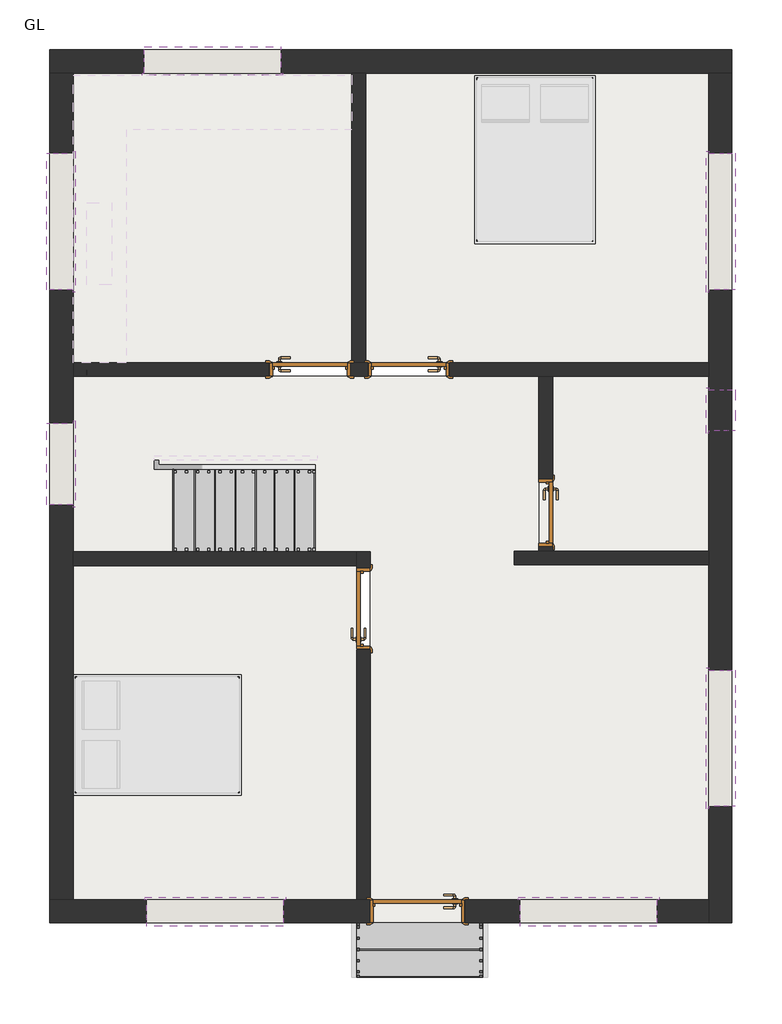
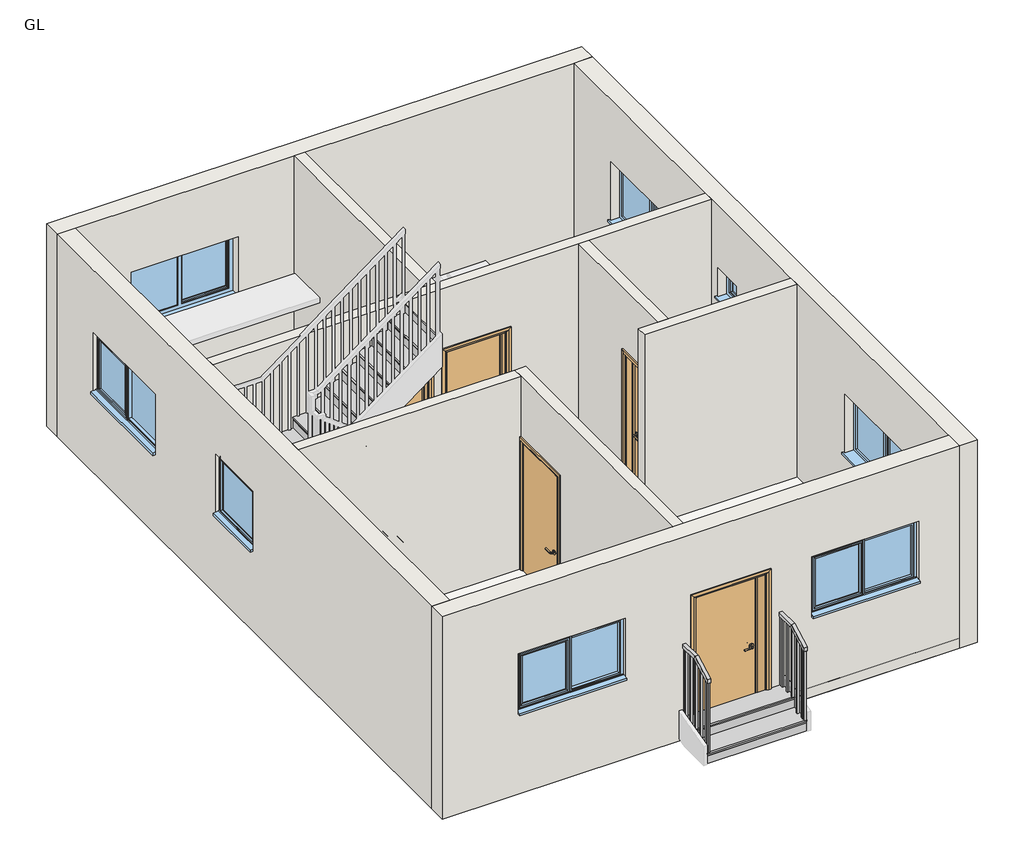
# One storey, part 1 of 2: 10 walls, 8 windows, 5 doors, 4 slabs, 2 railings, 2 stair flights.
"""IFC4 building model written with IfcOpenShell, lengths in millimetres."""

from ifc_helpers import new_model, si_unit, frame, origin, origin_with_axes, place, context, project, spatial, polyline, outline, extrude, faceted_brep, transform, mapped, element, save
from components import doors_intsgl_d1_0a18db40, doors_intsgl_d2_6b78dd6f, doors_intsgl_d2_f2c4d474, doors_intsgl_d3_2a6a78d5, wood_steps_w_50mm_tread_10mm_nosing_13mm_riser_f1b6b8d3, wood_steps_w_50mm_tread_10mm_nosing_13mm_riser_33fa0412, windows_dbl_plain_w1_b9c38b89, windows_sgl_plain_w2_7fc3d610, windows_sgl_plain_w3_b14593de

model = new_model("IFC4")

# Units and contexts
model_context = context("Model", 3, world=origin())
ifc_project = project(units=[si_unit("LENGTHUNIT", "METRE", prefix="MILLI")], contexts=[model_context])

# Site, building, storey
site = spatial("IfcSite", under=ifc_project)
building = spatial("IfcBuilding", under=site)
storey = spatial("IfcBuildingStorey", under=building, Name="GL", Elevation=0.0)

# Doors
placement = place(None, origin())
doors_intsgl_d1_shape = doors_intsgl_d1_0a18db40(model_context)
element("IfcDoor", 1, ObjectType="Doors_IntSgl : D1", at=placement, inside=storey, context=model_context, shape_type="MappedRepresentation", body=[
    mapped(doors_intsgl_d1_shape, transform((5070.9747157, 1805.1872041, 0.0), x_axis=(-1.0, 0.0, 0.0), y_axis=(0.0, -1.0, 0.0), z_axis=(0.0, 0.0, 1.0))),
])
doors_intsgl_d2_shape = doors_intsgl_d2_6b78dd6f(model_context)
element("IfcDoor", 2, ObjectType="Doors_IntSgl : D2", at=placement, inside=storey, context=model_context, shape_type="MappedRepresentation", body=[
    mapped(doors_intsgl_d2_shape, transform((4469.8879225, 5185.9272041, 0.0), x_axis=(0.0, 1.0, 0.0), y_axis=(-1.0, 0.0, 0.0), z_axis=(0.0, 0.0, 1.0))),
])
element("IfcDoor", 3, ObjectType="Doors_IntSgl : D2", at=placement, inside=storey, context=model_context, shape_type="MappedRepresentation", body=[
    mapped(doors_intsgl_d2_shape, transform((3869.5280726, 7859.2853898, 0.0), x_axis=(1.0, 0.0, 0.0), y_axis=(0.0, 1.0, 0.0), z_axis=(0.0, 0.0, 1.0))),
])
doors_intsgl_d2_2_shape = doors_intsgl_d2_f2c4d474(model_context)
element("IfcDoor", 4, ObjectType="Doors_IntSgl : D2", at=placement, inside=storey, context=model_context, shape_type="MappedRepresentation", body=[
    mapped(doors_intsgl_d2_2_shape, transform((4974.2756751, 7859.2853898, 0.0), x_axis=(-1.0, 0.0, 0.0), y_axis=(0.0, -1.0, 0.0), z_axis=(0.0, 0.0, 1.0))),
])
doors_intsgl_d3_shape = doors_intsgl_d3_2a6a78d5(model_context)
element("IfcDoor", 5, ObjectType="Doors_IntSgl : D3", at=placement, inside=storey, context=model_context, shape_type="MappedRepresentation", body=[
    mapped(doors_intsgl_d3_shape, transform((6504.4279225, 6259.0853898, 0.0), x_axis=(0.0, -1.0, 0.0), y_axis=(1.0, 0.0, 0.0), z_axis=(0.0, 0.0, 1.0))),
])

# Railings
element("IfcRailing", 6, ObjectType="1100mm", at=placement, inside=storey, context=model_context, shape_type="SolidModel", body=[
    faceted_brep([(5757.1747157, 1066.0472041, 1269.3333333), (5757.1747157, 1066.0472041, 1212.1353881), (5807.1747157, 1066.0472041, 1212.1353881), (5807.1747157, 1066.0472041, 1269.3333333), (5757.1747157, 1370.8472041, 1438.6666667), (5757.1747157, 1383.8035055, 1388.6666667), (5807.1747157, 1383.8035055, 1388.6666667), (5807.1747157, 1370.8472041, 1438.6666667), (5757.1747157, 1675.6472041, 1438.6666667), (5807.1747157, 1675.6472041, 1438.6666667), (5807.1747157, 1675.6472041, 1388.6666667), (5757.1747157, 1675.6472041, 1388.6666667)], [[[0, 1, 2, 3]], [[1, 0, 4, 5]], [[2, 1, 5, 6]], [[3, 2, 6, 7]], [[0, 3, 7, 4]], [[8, 9, 10, 11]], [[5, 4, 8, 11]], [[6, 5, 11, 10]], [[7, 6, 10, 9]], [[4, 7, 9, 8]]]),
    extrude(outline(polyline([(5794.6747157, 1616.0472041), (5769.6747157, 1616.0472041), (5769.6747157, 1641.0472041), (5794.6747157, 1641.0472041), (5794.6747157, 1616.0472041)])), frame((0.0, 0.0, 338.6666667), z_axis=(0.0, 0.0, 1.0), x_axis=(1.0, 0.0, 0.0)), (0.0, 0.0, 1.0), 1050.0),
    extrude(outline(polyline([(5794.6747157, 1491.0472041), (5769.6747157, 1491.0472041), (5769.6747157, 1516.0472041), (5794.6747157, 1516.0472041), (5794.6747157, 1491.0472041)])), frame((0.0, 0.0, 338.6666667), z_axis=(0.0, 0.0, 1.0), x_axis=(1.0, 0.0, 0.0)), (0.0, 0.0, 1.0), 1050.0),
    extrude(outline(polyline([(5794.6747157, 1366.0472041), (5769.6747157, 1366.0472041), (5769.6747157, 1391.0472041), (5794.6747157, 1391.0472041), (5794.6747157, 1366.0472041)])), frame((0.0, 0.0, 338.6666667), z_axis=(0.0, 0.0, 1.0), x_axis=(1.0, 0.0, 0.0)), (0.0, 0.0, 1.0), 1050.0),
    extrude(outline(polyline([(1241.0472041, 169.3333333), (1241.0472041, 1309.3576103), (1266.0472041, 1323.2464992), (1266.0472041, 169.3333333), (1241.0472041, 169.3333333)])), frame((5769.6747157, 0.0, 0.0), z_axis=(1.0, 0.0, 0.0), x_axis=(0.0, 1.0, 0.0)), (0.0, 0.0, 1.0), 25.0),
    extrude(outline(polyline([(1116.0472041, 169.3333333), (1116.0472041, 1239.9131659), (1141.0472041, 1253.8020548), (1141.0472041, 169.3333333), (1116.0472041, 169.3333333)])), frame((5769.6747157, 0.0, 0.0), z_axis=(1.0, 0.0, 0.0), x_axis=(0.0, 1.0, 0.0)), (0.0, 0.0, 1.0), 25.0),
    extrude(outline(polyline([(5794.6747157, 1650.6472041), (5769.6747157, 1650.6472041), (5769.6747157, 1675.6472041), (5794.6747157, 1675.6472041), (5794.6747157, 1650.6472041)])), frame((0.0, 0.0, 338.6666667), z_axis=(0.0, 0.0, 1.0), x_axis=(1.0, 0.0, 0.0)), (0.0, 0.0, 1.0), 1050.0),
    extrude(outline(polyline([(1066.0472041, 169.3333333), (1066.0472041, 1212.1353881), (1091.0472041, 1226.024277), (1091.0472041, 169.3333333), (1066.0472041, 169.3333333)])), frame((5769.6747157, 0.0, 0.0), z_axis=(1.0, 0.0, 0.0), x_axis=(0.0, 1.0, 0.0)), (0.0, 0.0, 1.0), 25.0),
])
element("IfcRailing", 7, ObjectType="1100mm", at=placement, inside=storey, context=model_context, shape_type="SolidModel", body=[
    faceted_brep([(4385.5747157, 1066.0472041, 1269.3333333), (4385.5747157, 1066.0472041, 1212.1353881), (4435.5747157, 1066.0472041, 1212.1353881), (4435.5747157, 1066.0472041, 1269.3333333), (4385.5747157, 1370.8472041, 1438.6666667), (4385.5747157, 1383.8035055, 1388.6666667), (4435.5747157, 1383.8035055, 1388.6666667), (4435.5747157, 1370.8472041, 1438.6666667), (4385.5747157, 1675.6472041, 1438.6666667), (4435.5747157, 1675.6472041, 1438.6666667), (4435.5747157, 1675.6472041, 1388.6666667), (4385.5747157, 1675.6472041, 1388.6666667)], [[[0, 1, 2, 3]], [[1, 0, 4, 5]], [[2, 1, 5, 6]], [[3, 2, 6, 7]], [[0, 3, 7, 4]], [[8, 9, 10, 11]], [[5, 4, 8, 11]], [[6, 5, 11, 10]], [[7, 6, 10, 9]], [[4, 7, 9, 8]]]),
    extrude(outline(polyline([(4398.0747157, 1616.0472041), (4398.0747157, 1641.0472041), (4423.0747157, 1641.0472041), (4423.0747157, 1616.0472041), (4398.0747157, 1616.0472041)])), frame((0.0, 0.0, 338.6666667), z_axis=(0.0, 0.0, 1.0), x_axis=(1.0, 0.0, 0.0)), (0.0, 0.0, 1.0), 1050.0),
    extrude(outline(polyline([(4398.0747157, 1491.0472041), (4398.0747157, 1516.0472041), (4423.0747157, 1516.0472041), (4423.0747157, 1491.0472041), (4398.0747157, 1491.0472041)])), frame((0.0, 0.0, 338.6666667), z_axis=(0.0, 0.0, 1.0), x_axis=(1.0, 0.0, 0.0)), (0.0, 0.0, 1.0), 1050.0),
    extrude(outline(polyline([(4398.0747157, 1366.0472041), (4398.0747157, 1391.0472041), (4423.0747157, 1391.0472041), (4423.0747157, 1366.0472041), (4398.0747157, 1366.0472041)])), frame((0.0, 0.0, 338.6666667), z_axis=(0.0, 0.0, 1.0), x_axis=(1.0, 0.0, 0.0)), (0.0, 0.0, 1.0), 1050.0),
    extrude(outline(polyline([(1241.0472041, 1309.3576103), (1266.0472041, 1323.2464992), (1266.0472041, 169.3333333), (1241.0472041, 169.3333333), (1241.0472041, 1309.3576103)])), frame((4398.0747157, 0.0, 0.0), z_axis=(1.0, 0.0, 0.0), x_axis=(0.0, 1.0, 0.0)), (0.0, 0.0, 1.0), 25.0),
    extrude(outline(polyline([(1116.0472041, 1239.9131659), (1141.0472041, 1253.8020548), (1141.0472041, 169.3333333), (1116.0472041, 169.3333333), (1116.0472041, 1239.9131659)])), frame((4398.0747157, 0.0, 0.0), z_axis=(1.0, 0.0, 0.0), x_axis=(0.0, 1.0, 0.0)), (0.0, 0.0, 1.0), 25.0),
    extrude(outline(polyline([(4398.0747157, 1650.6472041), (4398.0747157, 1675.6472041), (4423.0747157, 1675.6472041), (4423.0747157, 1650.6472041), (4398.0747157, 1650.6472041)])), frame((0.0, 0.0, 338.6666667), z_axis=(0.0, 0.0, 1.0), x_axis=(1.0, 0.0, 0.0)), (0.0, 0.0, 1.0), 1050.0),
    extrude(outline(polyline([(1066.0472041, 1212.1353881), (1091.0472041, 1226.024277), (1091.0472041, 169.3333333), (1066.0472041, 169.3333333), (1066.0472041, 1212.1353881)])), frame((4398.0747157, 0.0, 0.0), z_axis=(1.0, 0.0, 0.0), x_axis=(0.0, 1.0, 0.0)), (0.0, 0.0, 1.0), 25.0),
])

# Slabs
element("IfcSlab", 8, ObjectType="BEDROOM FLOORING", at=placement, inside=storey, context=model_context, shape_type="SweptSolid", body=[
    extrude(outline(polyline([(4393.6879225, 5668.5272041), (4393.6879225, 1934.7272041), (1223.7679225, 1934.7272041), (1223.7679225, 5668.5272041), (4393.6879225, 5668.5272041)])), origin_with_axes(), (0.0, 0.0, 1.0), 149.9616),
    extrude(outline(polyline([(8325.6079225, 11170.1672041), (8325.6079225, 7935.4853898), (4491.6756751, 7935.4853898), (4491.6756751, 11170.1672041), (8325.6079225, 11170.1672041)])), origin_with_axes(), (0.0, 0.0, 1.0), 149.9616),
])
element("IfcSlab", 9, ObjectType="HALL FLOORING", at=placement, inside=storey, context=model_context, shape_type="SweptSolid", body=[
    extrude(outline(polyline([(6428.2279225, 7783.0853898), (6428.2279225, 5827.2853898), (6155.5280726, 5827.2853898), (6155.5280726, 5700.2853898), (8325.6079225, 5700.2853898), (8325.6079225, 1675.6472041), (4546.0879225, 1675.6472041), (4546.0879225, 5820.9272041), (1223.7679225, 5820.9272041), (1223.7679225, 7783.0853898), (6428.2279225, 7783.0853898)])), origin_with_axes(), (0.0, 0.0, 1.0), 149.9616),
])
element("IfcSlab", 10, ObjectType="KITCHEN FLOORING", at=placement, inside=storey, context=model_context, shape_type="SweptSolid", body=[
    extrude(outline(polyline([(4361.7280726, 11170.1672041), (4361.7280726, 7935.4853898), (1223.7679225, 7935.4853898), (1223.7679225, 11170.1672041), (4361.7280726, 11170.1672041)])), origin_with_axes(), (0.0, 0.0, 1.0), 149.9616),
])
element("IfcSlab", 11, ObjectType="TOILET FLOORING", at=placement, inside=storey, context=model_context, shape_type="SweptSolid", body=[
    extrude(outline(polyline([(8325.6079225, 7783.0853898), (8325.6079225, 5827.2853898), (6428.2279225, 5827.2853898), (6428.2279225, 7783.0853898), (8325.6079225, 7783.0853898)])), origin_with_axes(), (0.0, 0.0, 1.0), 149.9616),
])

# Stair flights
wood_steps_w_50mm_tread_10mm_nosing_13mm_riser_shape = wood_steps_w_50mm_tread_10mm_nosing_13mm_riser_f1b6b8d3(model_context)
element("IfcStairFlight", 12, ObjectType="Wood_Steps_w-50mm_Tread-10mm_Nosing-13mm_Riser", at=placement, inside=storey, context=model_context, shape_type="MappedRepresentation", body=[
    mapped(wood_steps_w_50mm_tread_10mm_nosing_13mm_riser_shape, transform((0.0, 0.0, 0.0), x_axis=(1.0, 0.0, 0.0), y_axis=(0.0, 1.0, 0.0), z_axis=(0.0, 0.0, 1.0))),
])
wood_steps_w_50mm_tread_10mm_nosing_13mm_riser_2_shape = wood_steps_w_50mm_tread_10mm_nosing_13mm_riser_33fa0412(model_context)
element("IfcStairFlight", 13, ObjectType="Wood_Steps_w-50mm_Tread-10mm_Nosing-13mm_Riser", at=placement, inside=storey, context=model_context, shape_type="MappedRepresentation", body=[
    mapped(wood_steps_w_50mm_tread_10mm_nosing_13mm_riser_2_shape, transform((0.0, 0.0, 0.0), x_axis=(1.0, 0.0, 0.0), y_axis=(0.0, 1.0, 0.0), z_axis=(0.0, 0.0, 1.0))),
])

# Walls
element("IfcWall", 14, ObjectType="EXT WALL", at=placement, inside=storey, context=model_context, shape_type="Brep", body=[
    faceted_brep([(964.6879225, 11170.1672041, 0.0), (1223.7679225, 11170.1672041, 0.0), (4339.2756751, 11170.1672041, 0.0), (4491.6756751, 11170.1672041, 0.0), (8325.6079225, 11170.1672041, 0.0), (8584.6879225, 11170.1672041, 0.0), (8584.6879225, 11170.1672041, 3048.0), (8325.6079225, 11170.1672041, 3048.0), (4491.6756751, 11170.1672041, 3048.0), (4339.2756751, 11170.1672041, 3048.0), (1223.7679225, 11170.1672041, 3048.0), (964.6879225, 11170.1672041, 3048.0), (2019.5217988, 11170.1672041, 2110.0), (3543.5217988, 11170.1672041, 2110.0), (3543.5217988, 11170.1672041, 1200.0), (2019.5217988, 11170.1672041, 1200.0), (964.6879225, 11429.2472041, 0.0), (964.6879225, 11429.2472041, 3048.0), (8584.6879225, 11429.2472041, 3048.0), (8584.6879225, 11429.2472041, 0.0), (2019.5217988, 11429.2472041, 2110.0), (2019.5217988, 11429.2472041, 1200.0), (3543.5217988, 11429.2472041, 1200.0), (3543.5217988, 11429.2472041, 2110.0)], [[[0, 1, 2, 3, 4, 5, 6, 7, 8, 9, 10, 11], [12, 13, 14, 15]], [[16, 17, 18, 19], [20, 21, 22, 23]], [[5, 4, 3, 2, 1, 0, 16, 19]], [[11, 10, 9, 8, 7, 6, 18, 17]], [[6, 5, 19, 18]], [[0, 11, 17, 16]], [[21, 20, 12, 15]], [[22, 21, 15, 14]], [[23, 22, 14, 13]], [[20, 23, 13, 12]]]),
])
element("IfcWall", 15, ObjectType="EXT WALL", at=placement, inside=storey, context=model_context, shape_type="Brep", body=[
    faceted_brep([(8325.6079225, 11170.1672041, 0.0), (8325.6079225, 7935.4853898, 0.0), (8325.6079225, 7783.0853898, 0.0), (8325.6079225, 5827.2853898, 0.0), (8325.6079225, 5674.8853898, 0.0), (8325.6079225, 1934.7272041, 0.0), (8325.6079225, 1675.6472041, 0.0), (8325.6079225, 1675.6472041, 3048.0), (8325.6079225, 1934.7272041, 3048.0), (8325.6079225, 5674.8853898, 3048.0), (8325.6079225, 5827.2853898, 3048.0), (8325.6079225, 7783.0853898, 3048.0), (8325.6079225, 7935.4853898, 3048.0), (8325.6079225, 11170.1672041, 3048.0), (8325.6079225, 4500.1272041, 2110.0), (8325.6079225, 2976.1272041, 2110.0), (8325.6079225, 2976.1272041, 1200.0), (8325.6079225, 4500.1272041, 1200.0), (8325.6079225, 10272.2853898, 2110.0), (8325.6079225, 8748.2853898, 2110.0), (8325.6079225, 8748.2853898, 1200.0), (8325.6079225, 10272.2853898, 1200.0), (8325.6079225, 7630.6853898, 2110.0), (8325.6079225, 7173.4853898, 2110.0), (8325.6079225, 7173.4853898, 1652.8), (8325.6079225, 7630.6853898, 1652.8), (8584.6879225, 11170.1672041, 0.0), (8584.6879225, 11170.1672041, 3048.0), (8584.6879225, 1675.6472041, 3048.0), (8584.6879225, 1675.6472041, 0.0), (8584.6879225, 4500.1272041, 2110.0), (8584.6879225, 4500.1272041, 1200.0), (8584.6879225, 2976.1272041, 1200.0), (8584.6879225, 2976.1272041, 2110.0), (8584.6879225, 10272.2853898, 2110.0), (8584.6879225, 10272.2853898, 1200.0), (8584.6879225, 8748.2853898, 1200.0), (8584.6879225, 8748.2853898, 2110.0), (8584.6879225, 7630.6853898, 2110.0), (8584.6879225, 7630.6853898, 1652.8), (8584.6879225, 7173.4853898, 1652.8), (8584.6879225, 7173.4853898, 2110.0)], [[[0, 1, 2, 3, 4, 5, 6, 7, 8, 9, 10, 11, 12, 13], [14, 15, 16, 17], [18, 19, 20, 21], [22, 23, 24, 25]], [[26, 27, 28, 29], [30, 31, 32, 33], [34, 35, 36, 37], [38, 39, 40, 41]], [[6, 5, 4, 3, 2, 1, 0, 26, 29]], [[13, 12, 11, 10, 9, 8, 7, 28, 27]], [[0, 13, 27, 26]], [[7, 6, 29, 28]], [[31, 30, 14, 17]], [[32, 31, 17, 16]], [[33, 32, 16, 15]], [[30, 33, 15, 14]], [[35, 34, 18, 21]], [[36, 35, 21, 20]], [[37, 36, 20, 19]], [[34, 37, 19, 18]], [[39, 38, 22, 25]], [[40, 39, 25, 24]], [[41, 40, 24, 23]], [[38, 41, 23, 22]]]),
])
element("IfcWall", 16, ObjectType="EXT WALL", at=placement, inside=storey, context=model_context, shape_type="Brep", body=[
    faceted_brep([(964.6879225, 1934.7272041, 3048.0), (1223.7679225, 1934.7272041, 3048.0), (4393.6879225, 1934.7272041, 3048.0), (4546.0879225, 1934.7272041, 3048.0), (8325.6079225, 1934.7272041, 3048.0), (8325.6079225, 1934.7272041, 0.0), (5604.3747157, 1934.7272041, 0.0), (5604.3747157, 1934.7272041, 2110.0), (4537.5747157, 1934.7272041, 2110.0), (4537.5747157, 1934.7272041, 0.0), (4393.6879225, 1934.7272041, 0.0), (1223.7679225, 1934.7272041, 0.0), (964.6879225, 1934.7272041, 0.0), (3572.3747157, 1934.7272041, 2110.0), (2048.3747157, 1934.7272041, 2110.0), (2048.3747157, 1934.7272041, 1200.0), (3572.3747157, 1934.7272041, 1200.0), (7746.4879225, 1934.7272041, 2110.0), (6222.4879225, 1934.7272041, 2110.0), (6222.4879225, 1934.7272041, 1200.0), (7746.4879225, 1934.7272041, 1200.0), (8325.6079225, 1675.6472041, 3048.0), (964.6879225, 1675.6472041, 3048.0), (964.6879225, 1675.6472041, 0.0), (4537.5747157, 1675.6472041, 0.0), (4537.5747157, 1675.6472041, 2110.0), (5604.3747157, 1675.6472041, 2110.0), (5604.3747157, 1675.6472041, 0.0), (8325.6079225, 1675.6472041, 0.0), (3572.3747157, 1675.6472041, 2110.0), (3572.3747157, 1675.6472041, 1200.0), (2048.3747157, 1675.6472041, 1200.0), (2048.3747157, 1675.6472041, 2110.0), (7746.4879225, 1675.6472041, 2110.0), (7746.4879225, 1675.6472041, 1200.0), (6222.4879225, 1675.6472041, 1200.0), (6222.4879225, 1675.6472041, 2110.0)], [[[0, 1, 2, 3, 4, 5, 6, 7, 8, 9, 10, 11, 12], [13, 14, 15, 16], [17, 18, 19, 20]], [[21, 22, 23, 24, 25, 26, 27, 28], [29, 30, 31, 32], [33, 34, 35, 36]], [[5, 28, 27, 6]], [[23, 12, 11, 10, 9, 24]], [[4, 3, 2, 1, 0, 22, 21]], [[5, 4, 21, 28]], [[0, 12, 23, 22]], [[8, 25, 24, 9]], [[25, 8, 7, 26]], [[26, 7, 6, 27]], [[30, 29, 13, 16]], [[31, 30, 16, 15]], [[32, 31, 15, 14]], [[29, 32, 14, 13]], [[34, 33, 17, 20]], [[35, 34, 20, 19]], [[36, 35, 19, 18]], [[33, 36, 18, 17]]]),
])
element("IfcWall", 17, ObjectType="EXT WALL", at=placement, inside=storey, context=model_context, shape_type="Brep", body=[
    faceted_brep([(1223.7679225, 1934.7272041, 0.0), (1223.7679225, 5668.5272041, 0.0), (1223.7679225, 5820.9272041, 0.0), (1223.7679225, 7783.0853898, 0.0), (1223.7679225, 7935.4853898, 0.0), (1223.7679225, 11170.1672041, 0.0), (1223.7679225, 11170.1672041, 3048.0), (1223.7679225, 7935.4853898, 3048.0), (1223.7679225, 7783.0853898, 3048.0), (1223.7679225, 5820.9272041, 3048.0), (1223.7679225, 5668.5272041, 3048.0), (1223.7679225, 1934.7272041, 3048.0), (1223.7679225, 8748.2853898, 2110.0), (1223.7679225, 10272.2853898, 2110.0), (1223.7679225, 10272.2853898, 1200.0), (1223.7679225, 8748.2853898, 1200.0), (1223.7679225, 6344.8062969, 2110.0), (1223.7679225, 7259.2062969, 2110.0), (1223.7679225, 7259.2062969, 1200.0), (1223.7679225, 6344.8062969, 1200.0), (964.6879225, 1934.7272041, 0.0), (964.6879225, 1934.7272041, 3048.0), (964.6879225, 11170.1672041, 3048.0), (964.6879225, 11170.1672041, 0.0), (964.6879225, 8748.2853898, 2110.0), (964.6879225, 8748.2853898, 1200.0), (964.6879225, 10272.2853898, 1200.0), (964.6879225, 10272.2853898, 2110.0), (964.6879225, 6344.8062969, 2110.0), (964.6879225, 6344.8062969, 1200.0), (964.6879225, 7259.2062969, 1200.0), (964.6879225, 7259.2062969, 2110.0)], [[[0, 1, 2, 3, 4, 5, 6, 7, 8, 9, 10, 11], [12, 13, 14, 15], [16, 17, 18, 19]], [[20, 21, 22, 23], [24, 25, 26, 27], [28, 29, 30, 31]], [[5, 4, 3, 2, 1, 0, 20, 23]], [[11, 10, 9, 8, 7, 6, 22, 21]], [[6, 5, 23, 22]], [[0, 11, 21, 20]], [[25, 24, 12, 15]], [[26, 25, 15, 14]], [[27, 26, 14, 13]], [[24, 27, 13, 12]], [[29, 28, 16, 19]], [[30, 29, 19, 18]], [[31, 30, 18, 17]], [[28, 31, 17, 16]]]),
])
element("IfcWall", 18, ObjectType="INT", at=placement, inside=storey, context=model_context, shape_type="Brep", body=[
    faceted_brep([(8325.6079225, 7783.0853898, 3048.0), (6580.6279225, 7783.0853898, 3048.0), (6428.2279225, 7783.0853898, 3048.0), (1223.7679225, 7783.0853898, 3048.0), (1223.7679225, 7783.0853898, 0.0), (3412.3280726, 7783.0853898, 0.0), (3412.3280726, 7783.0853898, 2110.0), (4326.7280726, 7783.0853898, 2110.0), (4326.7280726, 7783.0853898, 0.0), (4517.0756751, 7783.0853898, 0.0), (4517.0756751, 7783.0853898, 2110.0), (5431.4756751, 7783.0853898, 2110.0), (5431.4756751, 7783.0853898, 0.0), (6428.2279225, 7783.0853898, 0.0), (6580.6279225, 7783.0853898, 0.0), (8325.6079225, 7783.0853898, 0.0), (1223.7679225, 7935.4853898, 3048.0), (4339.2756751, 7935.4853898, 3048.0), (4491.6756751, 7935.4853898, 3048.0), (8325.6079225, 7935.4853898, 3048.0), (8325.6079225, 7935.4853898, 0.0), (5431.4756751, 7935.4853898, 0.0), (5431.4756751, 7935.4853898, 2110.0), (4517.0756751, 7935.4853898, 2110.0), (4517.0756751, 7935.4853898, 0.0), (4491.6756751, 7935.4853898, 0.0), (4339.2756751, 7935.4853898, 0.0), (4326.7280726, 7935.4853898, 0.0), (4326.7280726, 7935.4853898, 2110.0), (3412.3280726, 7935.4853898, 2110.0), (3412.3280726, 7935.4853898, 0.0), (1223.7679225, 7935.4853898, 0.0)], [[[0, 1, 2, 3, 4, 5, 6, 7, 8, 9, 10, 11, 12, 13, 14, 15]], [[16, 17, 18, 19, 20, 21, 22, 23, 24, 25, 26, 27, 28, 29, 30, 31]], [[4, 31, 30, 5]], [[20, 15, 14, 13, 12, 21]], [[8, 27, 26, 25, 24, 9]], [[3, 2, 1, 0, 19, 18, 17, 16]], [[0, 15, 20, 19]], [[4, 3, 16, 31]], [[7, 28, 27, 8]], [[28, 7, 6, 29]], [[29, 6, 5, 30]], [[23, 10, 9, 24]], [[10, 23, 22, 11]], [[11, 22, 21, 12]]]),
])
element("IfcWall", 19, ObjectType="INT", at=placement, inside=storey, context=model_context, shape_type="Brep", body=[
    faceted_brep([(4546.0879225, 5820.9272041, 3048.0), (4546.0879225, 1934.7272041, 3048.0), (4546.0879225, 1934.7272041, 0.0), (4546.0879225, 4728.7272041, 0.0), (4546.0879225, 4728.7272041, 2110.0), (4546.0879225, 5643.1272041, 2110.0), (4546.0879225, 5643.1272041, 0.0), (4546.0879225, 5820.9272041, 0.0), (4393.6879225, 1934.7272041, 3048.0), (4393.6879225, 5668.5272041, 3048.0), (4393.6879225, 5820.9272041, 3048.0), (4393.6879225, 5820.9272041, 0.0), (4393.6879225, 5668.5272041, 0.0), (4393.6879225, 5643.1272041, 0.0), (4393.6879225, 5643.1272041, 2110.0), (4393.6879225, 4728.7272041, 2110.0), (4393.6879225, 4728.7272041, 0.0), (4393.6879225, 1934.7272041, 0.0), (4537.5747157, 1934.7272041, 0.0)], [[[0, 1, 2, 3, 4, 5, 6, 7]], [[8, 9, 10, 11, 12, 13, 14, 15, 16, 17]], [[2, 18, 17, 16, 3]], [[11, 7, 6, 13, 12]], [[1, 0, 10, 9, 8]], [[2, 1, 8, 17, 18]], [[0, 7, 11, 10]], [[5, 14, 13, 6]], [[14, 5, 4, 15]], [[15, 4, 3, 16]]]),
])
element("IfcWall", 20, ObjectType="INT", at=placement, inside=storey, context=model_context, shape_type="SweptSolid", body=[
    extrude(outline(polyline([(1223.7679225, 5820.9272041), (4393.6879225, 5820.9272041), (4393.6879225, 5668.5272041), (1223.7679225, 5668.5272041), (1223.7679225, 5820.9272041)])), origin_with_axes(), (0.0, 0.0, 1.0), 3048.0),
])
element("IfcWall", 21, ObjectType="INT", at=placement, inside=storey, context=model_context, shape_type="SweptSolid", body=[
    extrude(outline(polyline([(4339.2756751, 7935.4853898), (4339.2756751, 11170.1672041), (4491.6756751, 11170.1672041), (4491.6756751, 7935.4853898), (4339.2756751, 7935.4853898)])), origin_with_axes(), (0.0, 0.0, 1.0), 3048.0),
])
element("IfcWall", 22, ObjectType="INT", at=placement, inside=storey, context=model_context, shape_type="SweptSolid", body=[
    extrude(outline(polyline([(5827.2853898, 3048.0), (7783.0853898, 3048.0), (7783.0853898, 0.0), (6640.0853898, 0.0), (6640.0853898, 2110.0), (5878.0853898, 2110.0), (5878.0853898, 0.0), (5827.2853898, 0.0), (5827.2853898, 3048.0)])), frame((6428.2279225, 0.0, 0.0), z_axis=(1.0, 0.0, 0.0), x_axis=(0.0, 1.0, 0.0)), (0.0, 0.0, 1.0), 152.4),
])
element("IfcWall", 23, ObjectType="INT", at=placement, inside=storey, context=model_context, shape_type="Brep", body=[
    faceted_brep([(6155.5280726, 5674.8853898, 0.0), (8325.6079225, 5674.8853898, 0.0), (8325.6079225, 5674.8853898, 3048.0), (6155.5280726, 5674.8853898, 3048.0), (6155.5280726, 5827.2853898, 0.0), (6155.5280726, 5827.2853898, 3048.0), (6428.2279225, 5827.2853898, 3048.0), (6580.6279225, 5827.2853898, 3048.0), (8325.6079225, 5827.2853898, 3048.0), (8325.6079225, 5827.2853898, 0.0), (6580.6279225, 5827.2853898, 0.0), (6428.2279225, 5827.2853898, 0.0)], [[[0, 1, 2, 3]], [[4, 5, 6, 7, 8, 9, 10, 11]], [[1, 0, 4, 11, 10, 9]], [[3, 2, 8, 7, 6, 5]], [[0, 3, 5, 4]], [[2, 1, 9, 8]]]),
])

# Windows
windows_dbl_plain_w1_shape = windows_dbl_plain_w1_b9c38b89(model_context)
element("IfcWindow", 24, ObjectType="Windows_Dbl_Plain : W1", at=placement, inside=storey, context=model_context, shape_type="MappedRepresentation", body=[
    mapped(windows_dbl_plain_w1_shape, transform((2525.3747157, 1813.6437719, 0.0), x_axis=(-1.0, 0.0, 0.0), y_axis=(0.0, -1.0, 0.0), z_axis=(0.0, 0.0, 1.0))),
])
element("IfcWindow", 25, ObjectType="Windows_Dbl_Plain : W1", at=placement, inside=storey, context=model_context, shape_type="MappedRepresentation", body=[
    mapped(windows_dbl_plain_w1_shape, transform((6699.4879225, 1813.6437719, 0.0), x_axis=(-1.0, 0.0, 0.0), y_axis=(0.0, -1.0, 0.0), z_axis=(0.0, 0.0, 1.0))),
])
element("IfcWindow", 26, ObjectType="Windows_Dbl_Plain : W1", at=placement, inside=storey, context=model_context, shape_type="MappedRepresentation", body=[
    mapped(windows_dbl_plain_w1_shape, transform((8446.6913547, 3453.1272041, 0.0), x_axis=(0.0, -1.0, 0.0), y_axis=(1.0, 0.0, 0.0), z_axis=(0.0, 0.0, 1.0))),
])
element("IfcWindow", 27, ObjectType="Windows_Dbl_Plain : W1", at=placement, inside=storey, context=model_context, shape_type="MappedRepresentation", body=[
    mapped(windows_dbl_plain_w1_shape, transform((8446.6913547, 9225.2853898, 0.0), x_axis=(0.0, -1.0, 0.0), y_axis=(1.0, 0.0, 0.0), z_axis=(0.0, 0.0, 1.0))),
])
element("IfcWindow", 28, ObjectType="Windows_Dbl_Plain : W1", at=placement, inside=storey, context=model_context, shape_type="MappedRepresentation", body=[
    mapped(windows_dbl_plain_w1_shape, transform((3066.5217988, 11291.2506362, 0.0), x_axis=(1.0, 0.0, 0.0), y_axis=(0.0, 1.0, 0.0), z_axis=(0.0, 0.0, 1.0))),
])
element("IfcWindow", 29, ObjectType="Windows_Dbl_Plain : W1", at=placement, inside=storey, context=model_context, shape_type="MappedRepresentation", body=[
    mapped(windows_dbl_plain_w1_shape, transform((1102.6844904, 9795.2853898, 0.0), x_axis=(0.0, 1.0, 0.0), y_axis=(-1.0, 0.0, 0.0), z_axis=(0.0, 0.0, 1.0))),
])
windows_sgl_plain_w2_shape = windows_sgl_plain_w2_7fc3d610(model_context)
element("IfcWindow", 30, ObjectType="Windows_Sgl_Plain : W2", at=placement, inside=storey, context=model_context, shape_type="MappedRepresentation", body=[
    mapped(windows_sgl_plain_w2_shape, transform((1102.6844904, 6802.0062969, 0.0), x_axis=(0.0, 1.0, 0.0), y_axis=(-1.0, 0.0, 0.0), z_axis=(0.0, 0.0, 1.0))),
])
windows_sgl_plain_w3_shape = windows_sgl_plain_w3_b14593de(model_context)
element("IfcWindow", 31, ObjectType="Windows_Sgl_Plain : W3", at=placement, inside=storey, context=model_context, shape_type="MappedRepresentation", body=[
    mapped(windows_sgl_plain_w3_shape, transform((8446.6913547, 7402.0853898, 0.0), x_axis=(0.0, -1.0, 0.0), y_axis=(1.0, 0.0, 0.0), z_axis=(0.0, 0.0, 1.0))),
])

save(model, "model.ifc")

# Revit data of these elements
# Type "Doors_IntSgl : D1"
#   Type Mark = "46"
#   Type Comments = "Internal Single"
#   Operation = "SingleSwingRight"
#   Manufacturer = "Revit"
#   Keynote = "L20"
#   Description = "Internal Single Door"
#   Analytic Construction = "Metal"
#   UnderCut = 0.026247 ft
#   Tolerance = 0.006562 ft
#   Thickness = 0.124672 ft
#   Thermal Resistance (R) = 0.270117 (m²·K)/W
#   Structural Tolerance = 0.026247 ft
#   StopDepth = 0.104987 ft
#   Stop Thickness = 0.062336 ft
#   Rough Width = 3.5 ft
#   Rough Height = 6.922572 ft
#   Height to Top Lock Rail = 3.28084 ft
#   Heat Transfer Coefficient (U) = 3.7021 W/(m²·K)
#   Handle Z Distance = 2.952756 ft
#   Handle X Distance = 0.246063 ft
#   Frame Thickness = 0.104987 ft
#   Door Panel Width = 3.224409 ft
#   Door Panel Thickness = 0.124672 ft
#   Door Panel Offset = 0.0 ft
#   Height = 6.922572 ft
#   Width = 3.5 ft
#   Door Panel Height = 6.75853 ft
#   Architrave Setback = 0.016404 ft
#   Vis - Ironmongery = yes
#   Material Ironmongery = Door - Handle
#   Material Frame = Door - Frame/Mullion (1)
#   Material Door = Door - Panel
#   Material Architrave = Door - Architrave
#   Visual Light Transmittance = 0
#   Solar Heat Gain Coefficient = 0
#   Function = (empty or 0)
#   Wall Closure = (empty or 0)
# Type "Doors_IntSgl : D2"
#   Type Mark = "47"
#   Type Comments = "Internal Single"
#   Operation = "SingleSwingRight"
#   Manufacturer = "Revit"
#   Keynote = "L20"
#   Description = "Internal Single Door"
#   Analytic Construction = "Metal"
#   UnderCut = 0.026247 ft
#   Tolerance = 0.006562 ft
#   Thickness = 0.124672 ft
#   Thermal Resistance (R) = 0.270117 (m²·K)/W
#   Structural Tolerance = 0.026247 ft
#   StopDepth = 0.104987 ft
#   Stop Thickness = 0.062336 ft
#   Rough Width = 3.0 ft
#   Rough Height = 6.922572 ft
#   Height to Top Lock Rail = 3.28084 ft
#   Heat Transfer Coefficient (U) = 3.7021 W/(m²·K)
#   Handle Z Distance = 2.952756 ft
#   Handle X Distance = 0.246063 ft
#   Frame Thickness = 0.104987 ft
#   Door Panel Width = 2.724409 ft
#   Door Panel Thickness = 0.124672 ft
#   Door Panel Offset = 0.0 ft
#   Height = 6.922572 ft
#   Width = 3.0 ft
#   Door Panel Height = 6.75853 ft
#   Architrave Setback = 0.016404 ft
#   Vis - Ironmongery = yes
#   Material Ironmongery = Door - Handle
#   Material Frame = Door - Frame/Mullion (1)
#   Material Door = Door - Panel
#   Material Architrave = Door - Architrave
#   Visual Light Transmittance = 0
#   Solar Heat Gain Coefficient = 0
#   Function = (empty or 0)
#   Wall Closure = (empty or 0)
# Type "Doors_IntSgl : D3"
#   Type Mark = "48"
#   Type Comments = "Internal Single"
#   Operation = "SingleSwingRight"
#   Manufacturer = "Revit"
#   Keynote = "L20"
#   Description = "Internal Single Door"
#   Analytic Construction = "Metal"
#   UnderCut = 0.026247 ft
#   Tolerance = 0.006562 ft
#   Thickness = 0.124672 ft
#   Thermal Resistance (R) = 0.270117 (m²·K)/W
#   Structural Tolerance = 0.026247 ft
#   StopDepth = 0.104987 ft
#   Stop Thickness = 0.062336 ft
#   Rough Width = 2.5 ft
#   Rough Height = 6.922572 ft
#   Height to Top Lock Rail = 3.28084 ft
#   Heat Transfer Coefficient (U) = 3.7021 W/(m²·K)
#   Handle Z Distance = 2.952756 ft
#   Handle X Distance = 0.246063 ft
#   Frame Thickness = 0.104987 ft
#   Door Panel Width = 2.224409 ft
#   Door Panel Thickness = 0.124672 ft
#   Door Panel Offset = 0.0 ft
#   Height = 6.922572 ft
#   Width = 2.5 ft
#   Door Panel Height = 6.75853 ft
#   Architrave Setback = 0.016404 ft
#   Vis - Ironmongery = yes
#   Material Ironmongery = Door - Handle
#   Material Frame = Door - Frame/Mullion (1)
#   Material Door = Door - Panel
#   Material Architrave = Door - Architrave
#   Visual Light Transmittance = 0
#   Solar Heat Gain Coefficient = 0
#   Function = (empty or 0)
#   Wall Closure = (empty or 0)
# Type "1100mm"
#   built-in parameter 1008612 = 0.019685 (stored number, unit not read)
#   built-in parameter 1008611 = 0.019685 (stored number, unit not read)
#   built-in parameter 1008609 = 0.902231 (stored number, unit not read)
#   built-in parameter 1008604 = 0.19685 (stored number, unit not read)
#   built-in parameter 1008603 = 0.164042 (stored number, unit not read)
#   Railing Height = 3.608924 ft
#   built-in parameter 1008630 = 2
#   built-in parameter 1008610 = 2
#   built-in parameter 1008608 = 1
#   built-in parameter 1008618 = Baluster_Square : 25mm
# Type "BEDROOM FLOORING"
#   Function = 0
#   Layers, outside or top first: 0.072 ft "Wood Sheathing, Chipboard" (function 5); 0.42 ft "Structure, Timber Joist/Rafter Layer" (function 1)
# Type "HALL FLOORING"
#   Function = 0
#   Layers, outside or top first: 0.072 ft "Wood Sheathing, Chipboard" (function 5); 0.42 ft "Structure, Timber Joist/Rafter Layer" (function 1)
# Type "KITCHEN FLOORING"
#   Function = 0
#   Layers, outside or top first: 0.072 ft "Wood Sheathing, Chipboard" (function 5); 0.42 ft "Structure, Timber Joist/Rafter Layer" (function 1)
# Type "TOILET FLOORING"
#   Function = 0
#   Layers, outside or top first: 0.072 ft "Wood Sheathing, Chipboard" (function 5); 0.42 ft "Structure, Timber Joist/Rafter Layer" (function 1)
# Type "EXT WALL"
#   Keynote = "F10"
#   Layers, outside or top first: 0.85 ft "Brick, Common" (function 1)
# Type "INT"
#   Keynote = "F10"
#   Layers, outside or top first: 0.5 ft "Brick, Common" (function 1)
# Type "Windows_Dbl_Plain : W1"
#   Type Mark = "56"
#   Operation = "DoublePanelVertical"
#   Construction Type Id = "GSP4R"
#   Manufacturer = "Revit"
#   Keynote = "L10"
#   Analytic Construction = "1/8 in Pilkington single glazing"
#   Wrap Layers (Ext) from Ext = 0.336286 ft
#   Wrap Layers (Int) from Ext = 0.582349 ft
#   Window Board Projection = 0.082021 ft
#   Window Board Extension = 0.082021 ft
#   Visual Light Transmittance = 0.9
#   Solar Heat Gain Coefficient = 0.78
#   Rough Width = 5.0 ft
#   Rough Height = 2.985564 ft
#   Height = 2.985564 ft
#   Width = 5.0 ft
#   Heat Transfer Coefficient (U) = 3.6886 W/(m²·K)
#   Glazing Thickness = 0.07874 ft
#   FrameOffset - External = 0.164042 ft
#   Frame Depth = 0.213255 ft
#   Default Head Height = 6.922572 ft
#   Cill Depth = 0.287073 ft
#   Cavity Closer Width = 0.164042 ft
#   Cavity Closer Offset from Ext = 0.336286 ft
#   Cavity Closer Depth = 0.278871 ft
#   Vis - Cavity Closers = yes
#   Define Thermal Properties by = 1
#   Material Trim = Window Frame
#   Material Glass = Glass
#   Material Frame = Window Frame
#   Wall Closure = (empty or 0)
# Type "Windows_Sgl_Plain : W2"
#   Type Mark = "57"
#   Operation = "SinglePanel"
#   Construction Type Id = "SGL"
#   Manufacturer = "Revit"
#   Keynote = "L10"
#   Analytic Construction = "Large single-glazed windows"
#   Wrap Layers (Ext) from Ext = 0.336286 ft
#   Wrap Layers (Int) from Ext = 0.582349 ft
#   Window Board Projection = 0.082021 ft
#   Window Board Extension = 0.082021 ft
#   Visual Light Transmittance = 0.9
#   Solar Heat Gain Coefficient = 0.86
#   Rough Width = 3.0 ft
#   Rough Height = 2.985564 ft
#   Height = 2.985564 ft
#   Width = 3.0 ft
#   Heat Transfer Coefficient (U) = 5.5617 W/(m²·K)
#   Glazing Thickness = 0.07874 ft
#   FrameOffset - External = 0.164042 ft
#   Frame Depth = 0.213255 ft
#   Default Head Height = 6.922572 ft
#   Cill Depth = 0.287073 ft
#   Cavity Closer Width = 0.164042 ft
#   Cavity Closer Offset from Ext = 0.336286 ft
#   Cavity Closer Depth = 0.278871 ft
#   Vis - Cavity Closers = yes
#   Define Thermal Properties by = 1
#   Material Trim = Window Frame
#   Material Glass = Glass
#   Material Frame = Window Frame
#   Wall Closure = (empty or 0)
# Type "Windows_Sgl_Plain : W3"
#   Type Mark = "58"
#   Operation = "SinglePanel"
#   Construction Type Id = "SGL"
#   Manufacturer = "Revit"
#   Keynote = "L10"
#   Analytic Construction = "Large single-glazed windows"
#   Wrap Layers (Ext) from Ext = 0.336286 ft
#   Wrap Layers (Int) from Ext = 0.582349 ft
#   Window Board Projection = 0.082021 ft
#   Window Board Extension = 0.082021 ft
#   Visual Light Transmittance = 0.9
#   Solar Heat Gain Coefficient = 0.86
#   Rough Width = 1.5 ft
#   Rough Height = 1.5 ft
#   Height = 1.5 ft
#   Width = 1.5 ft
#   Heat Transfer Coefficient (U) = 5.5617 W/(m²·K)
#   Glazing Thickness = 0.07874 ft
#   FrameOffset - External = 0.164042 ft
#   Frame Depth = 0.213255 ft
#   Default Head Height = 6.922572 ft
#   Cill Depth = 0.287073 ft
#   Cavity Closer Width = 0.164042 ft
#   Cavity Closer Offset from Ext = 0.336286 ft
#   Cavity Closer Depth = 0.278871 ft
#   Vis - Cavity Closers = yes
#   Define Thermal Properties by = 1
#   Material Trim = Window Frame
#   Material Glass = Glass
#   Material Frame = Window Frame
#   Wall Closure = (empty or 0)
# Element 1 (IfcDoor, "Doors_IntSgl : D1")
#   Phase Created = New Construction
#   Materials on its faces: "Door - Architrave", "Door - Handle", "Door - Frame/Mullion (1)", "Door - Panel"
# Elements 2, 3, 4 (IfcDoor, "Doors_IntSgl : D2")
#   Phase Created = New Construction
#   Materials on its faces: "Door - Architrave", "Door - Handle", "Door - Frame/Mullion (1)", "Door - Panel"
# Element 5 (IfcDoor, "Doors_IntSgl : D3")
#   Phase Created = New Construction
#   Materials on its faces: "Door - Architrave", "Door - Handle", "Door - Frame/Mullion (1)", "Door - Panel"
# Elements 6, 7 (IfcRailing, "1100mm")
#   Phase Created = New Construction
# Element 8 (IfcSlab, "BEDROOM FLOORING")
#   Height Offset From Level = 0.492 ft
#   Phase Created = New Construction
#   Materials on its faces: "Structure, Timber Joist/Rafter Layer", "Wood Sheathing, Chipboard"
# Element 9 (IfcSlab, "HALL FLOORING")
#   Height Offset From Level = 0.492 ft
#   Phase Created = New Construction
#   Materials on its faces: "Structure, Timber Joist/Rafter Layer", "Wood Sheathing, Chipboard"
# Element 10 (IfcSlab, "KITCHEN FLOORING")
#   Height Offset From Level = 0.492 ft
#   Phase Created = New Construction
#   Materials on its faces: "Structure, Timber Joist/Rafter Layer", "Wood Sheathing, Chipboard"
# Element 11 (IfcSlab, "TOILET FLOORING")
#   Height Offset From Level = 0.492 ft
#   Phase Created = New Construction
#   Materials on its faces: "Structure, Timber Joist/Rafter Layer", "Wood Sheathing, Chipboard"
# Elements 12, 13 (IfcStairFlight, "Wood_Steps_w-50mm_Tread-10mm_Nosing-13mm_Riser")
#   Phase Created = New Construction
#   Materials on its faces: "Oak Flooring"
# Elements 14, 15, 16, 17 (IfcWall, "EXT WALL")
#   Top Offset = 0.0 ft
#   Base Offset = 0.0 ft
#   wall height = 10.0 ft
#   Phase Created = New Construction
#   Base Constraint = GL
#   Top Constraint = FFL
#   Materials on its faces: "Brick, Common"
# Elements 18, 19, 20, 21, 22, 23 (IfcWall, "INT")
#   Top Offset = 0.0 ft
#   Base Offset = 0.0 ft
#   wall height = 10.0 ft
#   Phase Created = New Construction
#   Base Constraint = GL
#   Top Constraint = FFL
#   Materials on its faces: "Brick, Common"
# Element 24 (IfcWindow, "Windows_Dbl_Plain : W1")
#   Mark = "1"
#   Phase Created = New Construction
#   Materials on its faces: "Window Frame", "Glass"
# Element 25 (IfcWindow, "Windows_Dbl_Plain : W1")
#   Mark = "2"
#   Phase Created = New Construction
#   Materials on its faces: "Window Frame", "Glass"
# Element 26 (IfcWindow, "Windows_Dbl_Plain : W1")
#   Mark = "3"
#   Phase Created = New Construction
#   Materials on its faces: "Window Frame", "Glass"
# Element 27 (IfcWindow, "Windows_Dbl_Plain : W1")
#   Mark = "4"
#   Phase Created = New Construction
#   Materials on its faces: "Window Frame", "Glass"
# Element 28 (IfcWindow, "Windows_Dbl_Plain : W1")
#   Mark = "5"
#   Phase Created = New Construction
#   Materials on its faces: "Window Frame", "Glass"
# Element 29 (IfcWindow, "Windows_Dbl_Plain : W1")
#   Mark = "6"
#   Phase Created = New Construction
#   Materials on its faces: "Window Frame", "Glass"
# Element 30 (IfcWindow, "Windows_Sgl_Plain : W2")
#   Mark = "7"
#   Phase Created = New Construction
#   Materials on its faces: "Window Frame", "Glass"
# Element 31 (IfcWindow, "Windows_Sgl_Plain : W3")
#   Mark = "8"
#   Phase Created = New Construction
#   Materials on its faces: "Window Frame", "Glass"
# Materials
#   "Door - Handle": colour RGB 0 0 0, transparency 0, Keynote = "P21", Cost = 0
#   "Door - Frame/Mullion (1)": class "Wood", colour RGB 212 179 113, transparency 0, Keynote = "L20", Cost = 0
#   "Door - Panel": class "Wood", colour RGB 210 159 95, transparency 0, Keynote = "L20", Cost = 0
#   "Door - Architrave": class "Wood", colour RGB 154 90 5, transparency 0, Keynote = "P20", Cost = 0
#   "Wood Sheathing, Chipboard": class "Wood", colour RGB 127 127 127, transparency 0, Description = "Particleboard sheathing", Cost = 0
#   "Structure, Timber Joist/Rafter Layer": class "Wood", colour RGB 127 127 127, transparency 0, Description = "Timber framing, thermal airspace", Cost = 0
#   "Brick, Common": class "Masonry", colour RGB 170 100 105, transparency 0, Description = "Common brick", Cost = 0
#   "Window Frame": colour RGB 249 249 249, transparency 0, Keynote = "L10", Cost = 0
#   "Glass": class "Glass", colour RGB 0 128 192, transparency 0.9, Description = "Soda Lime Glass", Cost = 0
#   "Oak Flooring": class "Wood", colour RGB 212 179 113, transparency 0, Description = "Quercus Rubra", Cost = 0
